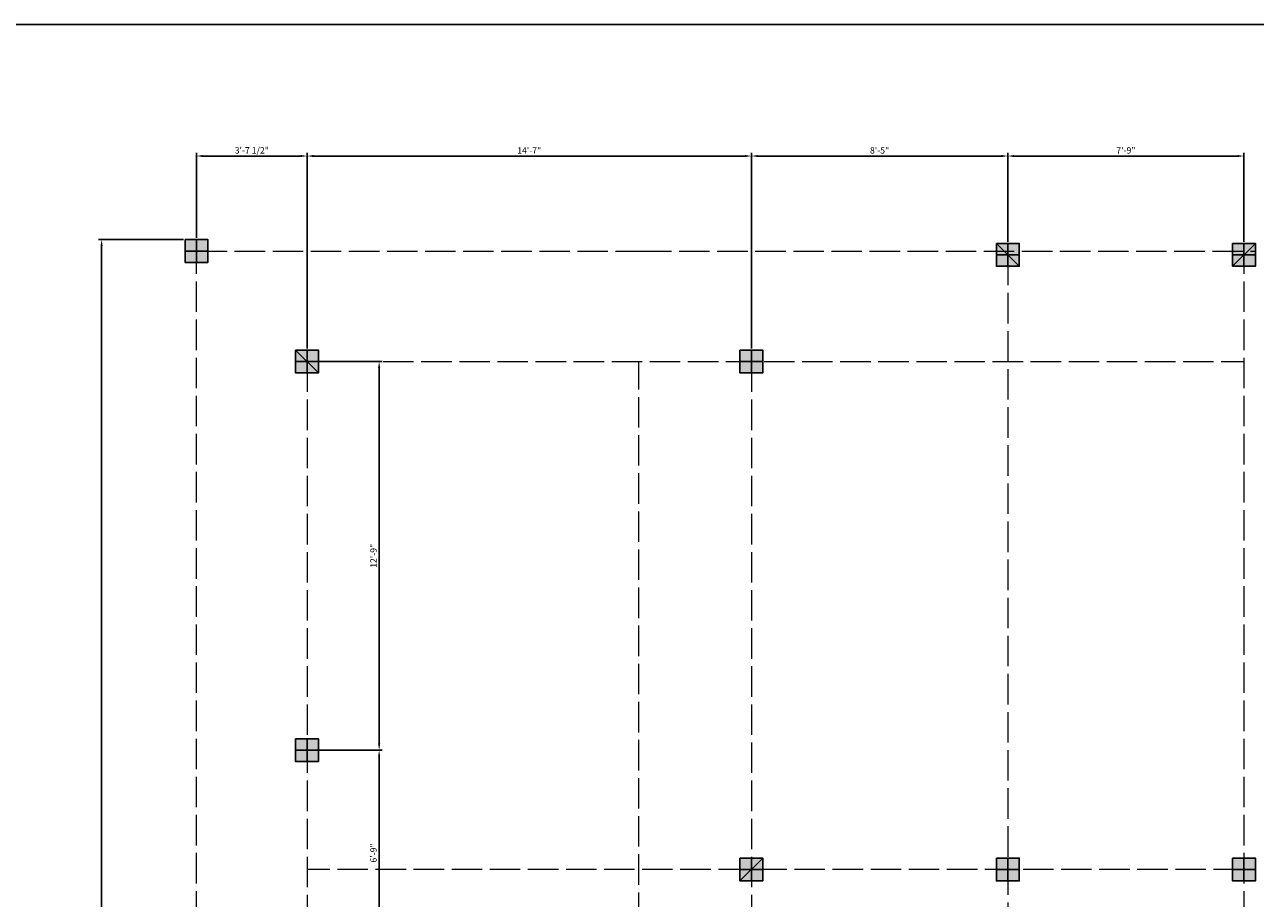
# Model space of a CAD drawing. Units: inches. Extents: x 2163 to 7246, y 928 to 2098.
# Tile 9 of 15: x 2706 to 3191, y 1754 to 2098. Entities that reach past the tile are written whole.
import ezdxf

# ---------------------------------------------------------------- set-up
doc = ezdxf.new("R2010")
doc.units = ezdxf.units.IN
doc.linetypes.add('ACAD_ISO02W100', pattern=[15, 12, -3])
for name, color, linetype, lineweight in [('A-ANNO-DIMS', 4, 'Continuous', 18), ('A-ANNO-TTLB', 7, 'Continuous', 30), ('A-COLS', 41, 'Continuous', 30), ('A-GRID', 1, 'ACAD_ISO02W100', 18)]:
    doc.layers.add(name, color=color, linetype=linetype, lineweight=lineweight)
doc.layers.add('A-COLS-PATT', color=51, linetype='Continuous', lineweight=9, true_color=0xf8f6b0)
doc.styles.get("Standard").update_dxf_attribs({"font": 'arial.ttf'})
doc.dimstyles.new('ISO-25', dxfattribs={"dimtxt": 2.5, "dimasz": 2.5, "dimexe": 1.25, "dimexo": 0.625, "dimtad": 1, "dimdec": 0, "dimlunit": 3, "dimtxsty": 'Standard', "dimcen": 2.5, "dimadec": 0, "dimazin": 0, "dimtfac": 1, "dimtdec": 0, "dimtmove": 0, "dimatfit": 3, "dimfxl": 1, "dimarcsym": 0})

# ---------------------------------------------------------------- blocks, each defined once
blk = doc.blocks.new('COL-9X9-CENTERED')
for p, q in [((4.5, 9), (4.5, 0)), ((0, 4.5), (9, 4.5))]:
    blk.add_line(p, q)
blk.add_lwpolyline([(0, 9), (9, 9), (9, 0), (0, 0)], close=True)
blk = doc.blocks.new('*D80')
at = {"layer": 'A-ANNO-DIMS', "color": 0, "lineweight": -2, "transparency": 16777216}
for p, q in [((2768.6, 2013.57), (2735.07, 2013.57)), ((2736.32, 2011.07), (2736.32, 1413.07)), ((2768.6, 1410.57), (2735.07, 1410.57))]:
    blk.add_line(p, q, dxfattribs=at)
at = {"layer": 'A-ANNO-DIMS', "color": 0, "transparency": 16777216}
for points in [[(2735.91, 2011.07), (2736.74, 2011.07), (2736.32, 2013.57)], [(2735.91, 1413.07), (2736.74, 1413.07), (2736.32, 1410.57)]]:
    blk.add_solid(points, dxfattribs=at)
at = {"layer": 'Defpoints', "color": 0, "transparency": 16777216}
for p in [(2769.22, 2013.57), (2736.32, 1410.57), (2769.22, 1410.57)]:
    blk.add_point(p, dxfattribs=at)
at = {"layer": 'A-ANNO-DIMS', "color": 0, "transparency": 16777216, "insert": (2734.42, 1712.07), "char_height": 2.5, "attachment_point": 5, "rotation": 90}
blk.add_mtext('50\'-3"', dxfattribs=at)
blk = doc.blocks.new('*D81')
at = {"layer": 'A-ANNO-DIMS', "color": 0, "lineweight": -2, "transparency": 16777216}
for p, q in [((2773.72, 2014.2), (2773.72, 2047.72)), ((2776.22, 2046.47), (2814.72, 2046.47)), ((2817.22, 1970.7), (2817.22, 2047.72))]:
    blk.add_line(p, q, dxfattribs=at)
at = {"layer": 'A-ANNO-DIMS', "color": 0, "transparency": 16777216}
for points in [[(2776.22, 2046.89), (2776.22, 2046.06), (2773.72, 2046.47)], [(2814.72, 2046.89), (2814.72, 2046.06), (2817.22, 2046.47)]]:
    blk.add_solid(points, dxfattribs=at)
at = {"layer": 'Defpoints', "color": 0, "transparency": 16777216}
for p in [(2817.22, 2046.47), (2773.72, 2013.57), (2817.22, 1970.07)]:
    blk.add_point(p, dxfattribs=at)
at = {"layer": 'A-ANNO-DIMS', "color": 0, "transparency": 16777216, "insert": (2795.47, 2048.39), "char_height": 2.5, "attachment_point": 5}
blk.add_mtext('3\'-7 1/2"', dxfattribs=at)
blk = doc.blocks.new('*D82')
at = {"layer": 'A-ANNO-DIMS', "color": 0, "lineweight": -2, "transparency": 16777216}
for p, q in [((2817.22, 1970.7), (2817.22, 2047.72)), ((2819.72, 2046.47), (2989.72, 2046.47)), ((2992.22, 1970.7), (2992.22, 2047.72))]:
    blk.add_line(p, q, dxfattribs=at)
at = {"layer": 'A-ANNO-DIMS', "color": 0, "transparency": 16777216}
for points in [[(2819.72, 2046.89), (2819.72, 2046.06), (2817.22, 2046.47)], [(2989.72, 2046.89), (2989.72, 2046.06), (2992.22, 2046.47)]]:
    blk.add_solid(points, dxfattribs=at)
at = {"layer": 'Defpoints', "color": 0, "transparency": 16777216}
for p in [(2992.22, 2046.47), (2817.22, 1970.07), (2992.22, 1970.07)]:
    blk.add_point(p, dxfattribs=at)
at = {"layer": 'A-ANNO-DIMS', "color": 0, "transparency": 16777216, "insert": (2904.72, 2048.35), "char_height": 2.5, "attachment_point": 5}
blk.add_mtext('14\'-7"', dxfattribs=at)
blk = doc.blocks.new('*D84')
at = {"layer": 'A-ANNO-DIMS', "color": 0, "lineweight": -2, "transparency": 16777216}
for p, q in [((2992.22, 1970.7), (2992.22, 2047.72)), ((2994.72, 2046.47), (3090.72, 2046.47)), ((3093.22, 2012.7), (3093.22, 2047.72))]:
    blk.add_line(p, q, dxfattribs=at)
at = {"layer": 'A-ANNO-DIMS', "color": 0, "transparency": 16777216}
for points in [[(2994.72, 2046.89), (2994.72, 2046.06), (2992.22, 2046.47)], [(3090.72, 2046.89), (3090.72, 2046.06), (3093.22, 2046.47)]]:
    blk.add_solid(points, dxfattribs=at)
at = {"layer": 'Defpoints', "color": 0, "transparency": 16777216}
for p in [(3093.22, 2046.47), (3093.22, 2012.07), (2992.22, 1970.07)]:
    blk.add_point(p, dxfattribs=at)
at = {"layer": 'A-ANNO-DIMS', "color": 0, "transparency": 16777216, "insert": (3042.72, 2048.37), "char_height": 2.5, "attachment_point": 5}
blk.add_mtext('8\'-5"', dxfattribs=at)
blk = doc.blocks.new('*D85')
at = {"layer": 'A-ANNO-DIMS', "color": 0, "lineweight": -2, "transparency": 16777216}
for p, q in [((3093.22, 2012.7), (3093.22, 2047.72)), ((3095.72, 2046.47), (3183.72, 2046.47)), ((3186.22, 2012.7), (3186.22, 2047.72))]:
    blk.add_line(p, q, dxfattribs=at)
at = {"layer": 'A-ANNO-DIMS', "color": 0, "transparency": 16777216}
for points in [[(3095.72, 2046.89), (3095.72, 2046.06), (3093.22, 2046.47)], [(3183.72, 2046.89), (3183.72, 2046.06), (3186.22, 2046.47)]]:
    blk.add_solid(points, dxfattribs=at)
at = {"layer": 'Defpoints', "color": 0, "transparency": 16777216}
for p in [(3186.22, 2046.47), (3093.22, 2012.07), (3186.22, 2012.07)]:
    blk.add_point(p, dxfattribs=at)
at = {"layer": 'A-ANNO-DIMS', "color": 0, "transparency": 16777216, "insert": (3139.72, 2048.37), "char_height": 2.5, "attachment_point": 5}
blk.add_mtext('7\'-9"', dxfattribs=at)
blk = doc.blocks.new('*D90')
at = {"layer": 'A-ANNO-DIMS', "color": 0, "lineweight": -2, "transparency": 16777216}
for p, q in [((2813.35, 1965.57), (2846.87, 1965.57)), ((2845.62, 1963.07), (2845.62, 1815.07)), ((2813.35, 1812.57), (2846.87, 1812.57))]:
    blk.add_line(p, q, dxfattribs=at)
at = {"layer": 'A-ANNO-DIMS', "color": 0, "transparency": 16777216}
for points in [[(2845.21, 1963.07), (2846.04, 1963.07), (2845.62, 1965.57)], [(2845.21, 1815.07), (2846.04, 1815.07), (2845.62, 1812.57)]]:
    blk.add_solid(points, dxfattribs=at)
at = {"layer": 'Defpoints', "color": 0, "transparency": 16777216}
for p in [(2812.72, 1965.57), (2812.72, 1812.57), (2845.62, 1812.57)]:
    blk.add_point(p, dxfattribs=at)
at = {"layer": 'A-ANNO-DIMS', "color": 0, "transparency": 16777216, "insert": (2843.72, 1889.07), "char_height": 2.5, "attachment_point": 5, "rotation": 90}
blk.add_mtext('12\'-9"', dxfattribs=at)
blk = doc.blocks.new('*D91')
at = {"layer": 'A-ANNO-DIMS', "color": 0, "lineweight": -2, "transparency": 16777216}
for p, q in [((2813.35, 1812.57), (2846.87, 1812.57)), ((2845.62, 1810.07), (2845.62, 1734.07)), ((2813.35, 1731.57), (2846.87, 1731.57))]:
    blk.add_line(p, q, dxfattribs=at)
at = {"layer": 'A-ANNO-DIMS', "color": 0, "transparency": 16777216}
for points in [[(2845.21, 1810.07), (2846.04, 1810.07), (2845.62, 1812.57)], [(2845.21, 1734.07), (2846.04, 1734.07), (2845.62, 1731.57)]]:
    blk.add_solid(points, dxfattribs=at)
at = {"layer": 'Defpoints', "color": 0, "transparency": 16777216}
for p in [(2812.72, 1812.57), (2812.72, 1731.57), (2845.62, 1731.57)]:
    blk.add_point(p, dxfattribs=at)
at = {"layer": 'A-ANNO-DIMS', "color": 0, "transparency": 16777216, "insert": (2843.72, 1772.07), "char_height": 2.5, "attachment_point": 5, "rotation": 90}
blk.add_mtext('6\'-9"', dxfattribs=at)

msp = doc.modelspace()

# ---------------------------------------------------------------- hatches: boundary and pattern name
at = {"layer": 'A-COLS-PATT'}
h = msp.add_hatch(color=256, dxfattribs=at)
h.dxf.hatch_style = 1
h.paths.add_polyline_path([(2778.22, 2009.07), (2773.72, 2009.07), (2773.72, 2004.57), (2778.22, 2004.57)])
h.paths.add_polyline_path([(2778.22, 2013.57), (2773.72, 2013.57), (2773.72, 2009.07), (2778.22, 2009.07)])
h.paths.add_polyline_path([(2773.72, 2013.57), (2769.22, 2013.57), (2769.22, 2009.07), (2773.72, 2009.07)])
h.paths.add_polyline_path([(2773.72, 2009.07), (2769.22, 2009.07), (2769.22, 2004.57), (2773.72, 2004.57)])
h.paths.add_polyline_path([(2817.22, 1965.57), (2812.72, 1965.57), (2812.72, 1961.07), (2817.22, 1961.07)])
h.paths.add_polyline_path([(2817.22, 1970.07), (2812.72, 1970.07), (2817.22, 1965.57)])
h.paths.add_polyline_path([(2821.72, 1965.57), (2817.22, 1965.57), (2821.72, 1961.07)], flags=17)
h.paths.add_polyline_path([(2817.22, 1965.57), (2817.22, 1961.07), (2821.72, 1961.07)], flags=17)
h.paths.add_polyline_path([(2821.72, 1970.07), (2817.22, 1970.07), (2817.22, 1965.57), (2821.72, 1965.57)])
h.paths.add_polyline_path([(2812.72, 1970.07), (2812.72, 1965.57), (2817.22, 1965.57)], flags=17)
h.paths.add_polyline_path([(2992.22, 1970.07), (2987.72, 1970.07), (2987.72, 1965.57), (2992.22, 1965.57)])
h.paths.add_polyline_path([(2996.72, 1970.07), (2992.22, 1970.07), (2992.22, 1965.57), (2996.72, 1965.57)])
h.paths.add_polyline_path([(2996.72, 1965.57), (2992.22, 1965.57), (2992.22, 1961.07), (2996.72, 1961.07)])
h.paths.add_polyline_path([(2992.22, 1965.57), (2987.72, 1965.57), (2987.72, 1961.07), (2992.22, 1961.07)])
h.paths.add_polyline_path([(3097.72, 2012.07), (3093.22, 2012.07), (3093.22, 2009.07), (3097.72, 2009.07)])
h.paths.add_polyline_path([(3093.22, 2012.07), (3088.72, 2012.07), (3091.72, 2009.07), (3093.22, 2009.07)])
h.paths.add_polyline_path([(3091.72, 2009.07), (3088.72, 2009.07), (3088.72, 2007.57), (3093.22, 2007.57)])
h.paths.add_polyline_path([(3088.72, 2012.07), (3088.72, 2009.07), (3091.72, 2009.07)])
h.paths.add_polyline_path([(3097.72, 2009.07), (3093.22, 2009.07), (3093.22, 2007.57), (3097.72, 2007.57)])
h.paths.add_polyline_path([(3093.22, 2009.07), (3091.72, 2009.07), (3093.22, 2007.57)], flags=17)
h.paths.add_polyline_path([(3093.22, 2007.57), (3088.72, 2007.57), (3088.72, 2003.07), (3093.22, 2003.07)])
h.paths.add_polyline_path([(3093.22, 2007.57), (3093.22, 2003.07), (3097.72, 2003.07)])
h.paths.add_polyline_path([(3097.72, 2007.57), (3093.22, 2007.57), (3097.72, 2003.07)], flags=17)
h.paths.add_polyline_path([(3186.22, 2012.07), (3181.72, 2012.07), (3181.72, 2009.07), (3186.22, 2009.07)])
h.paths.add_polyline_path([(3190.72, 2012.07), (3186.22, 2012.07), (3186.22, 2009.07), (3187.72, 2009.07)])
h.paths.add_polyline_path([(3190.72, 2012.07), (3187.72, 2009.07), (3190.72, 2009.07)], flags=17)
h.paths.add_polyline_path([(3190.72, 2009.07), (3187.72, 2009.07), (3186.22, 2007.57), (3190.72, 2007.57)])
h.paths.add_polyline_path([(3187.72, 2009.07), (3186.22, 2009.07), (3186.22, 2007.57)], flags=17)
h.paths.add_polyline_path([(3186.22, 2009.07), (3181.72, 2009.07), (3181.72, 2007.57), (3186.22, 2007.57)])
h.paths.add_polyline_path([(3186.22, 2007.57), (3181.72, 2007.57), (3181.72, 2003.07)], flags=17)
h.paths.add_polyline_path([(3186.22, 2007.57), (3181.72, 2003.07), (3186.22, 2003.07)], flags=17)
h.paths.add_polyline_path([(3190.72, 2007.57), (3186.22, 2007.57), (3186.22, 2003.07), (3190.72, 2003.07)])
h.paths.add_polyline_path([(2817.22, 1812.57), (2812.72, 1812.57), (2812.72, 1808.07), (2817.22, 1808.07)])
h.paths.add_polyline_path([(2817.22, 1817.07), (2812.72, 1817.07), (2812.72, 1812.57), (2817.22, 1812.57)])
h.paths.add_polyline_path([(2821.72, 1817.07), (2817.22, 1817.07), (2817.22, 1812.57), (2821.72, 1812.57)])
h.paths.add_polyline_path([(2821.72, 1812.57), (2817.22, 1812.57), (2817.22, 1808.07), (2821.72, 1808.07)])
h.paths.add_polyline_path([(2821.72, 1736.07), (2817.22, 1736.07), (2817.22, 1731.57), (2821.72, 1731.57)])
h.paths.add_polyline_path([(2817.22, 1736.07), (2812.72, 1736.07), (2812.72, 1731.57), (2817.22, 1731.57)])
h.paths.add_polyline_path([(2817.22, 1731.57), (2812.72, 1731.57), (2812.72, 1727.07), (2817.22, 1727.07)])
h.paths.add_polyline_path([(2821.72, 1731.57), (2817.22, 1731.57), (2817.22, 1727.07), (2821.72, 1727.07)])
h.paths.add_polyline_path([(2992.22, 1765.57), (2987.72, 1761.07), (2992.22, 1761.07)], flags=17)
h.paths.add_polyline_path([(2992.22, 1765.57), (2987.72, 1765.57), (2987.72, 1761.07)])
h.paths.add_polyline_path([(2992.22, 1770.07), (2987.72, 1770.07), (2987.72, 1765.57), (2992.22, 1765.57)])
h.paths.add_polyline_path([(2996.72, 1770.07), (2992.22, 1770.07), (2992.22, 1765.57)])
h.paths.add_polyline_path([(2996.72, 1770.07), (2992.22, 1765.57), (2996.72, 1765.57)], flags=17)
h.paths.add_polyline_path([(2996.72, 1765.57), (2992.22, 1765.57), (2992.22, 1761.07), (2996.72, 1761.07)])
h.paths.add_polyline_path([(3097.72, 1770.07), (3093.22, 1770.07), (3093.22, 1765.57), (3097.72, 1765.57)])
h.paths.add_polyline_path([(3093.22, 1770.07), (3088.72, 1770.07), (3088.72, 1765.57), (3093.22, 1765.57)])
h.paths.add_polyline_path([(3093.22, 1765.57), (3088.72, 1765.57), (3088.72, 1761.07), (3093.22, 1761.07)])
h.paths.add_polyline_path([(3097.72, 1765.57), (3093.22, 1765.57), (3093.22, 1761.07), (3097.72, 1761.07)])
h.paths.add_polyline_path([(3186.22, 1770.07), (3181.72, 1770.07), (3181.72, 1765.57), (3186.22, 1765.57)])
h.paths.add_polyline_path([(3190.72, 1770.07), (3186.22, 1770.07), (3186.22, 1765.57), (3190.72, 1765.57)])
h.paths.add_polyline_path([(3190.72, 1765.57), (3186.22, 1765.57), (3186.22, 1761.07), (3190.72, 1761.07)])
h.paths.add_polyline_path([(3186.22, 1765.57), (3181.72, 1765.57), (3181.72, 1761.07), (3186.22, 1761.07)])
h.paths.add_polyline_path([(2946.22, 1626.57), (2941.72, 1626.57), (2941.72, 1622.07), (2946.22, 1622.07)])
h.paths.add_polyline_path([(2946.22, 1631.07), (2941.72, 1631.07), (2941.72, 1626.57), (2946.22, 1626.57)])
h.paths.add_polyline_path([(2950.72, 1631.07), (2947.91, 1631.07), (2947.91, 1626.57), (2950.72, 1626.57)])
h.paths.add_polyline_path([(2947.91, 1631.07), (2946.22, 1631.07), (2946.22, 1626.57), (2947.91, 1626.57)])
h.paths.add_polyline_path([(2947.91, 1626.57), (2946.22, 1626.57), (2946.22, 1622.07), (2947.91, 1622.07)])
h.paths.add_polyline_path([(2950.72, 1626.57), (2947.91, 1626.57), (2947.91, 1622.07), (2950.72, 1622.07)])
h.paths.add_polyline_path([(2821.72, 1626.57), (2817.22, 1626.57), (2817.22, 1622.07), (2821.72, 1622.07)])
h.paths.add_polyline_path([(2821.72, 1631.07), (2817.22, 1626.57), (2821.72, 1626.57)])
h.paths.add_polyline_path([(2821.72, 1631.07), (2817.22, 1631.07), (2817.22, 1626.57)], flags=17)
h.paths.add_polyline_path([(2817.22, 1631.07), (2812.72, 1631.07), (2812.72, 1626.57), (2817.22, 1626.57)])
h.paths.add_polyline_path([(2817.22, 1626.57), (2812.72, 1626.57), (2812.72, 1622.07)], flags=17)
h.paths.add_polyline_path([(2817.22, 1626.57), (2812.72, 1622.07), (2817.22, 1622.07)])
h.paths.add_polyline_path([(3190.72, 1612.57), (3186.22, 1612.57), (3186.22, 1608.07), (3190.72, 1608.07)])
h.paths.add_polyline_path([(3186.22, 1612.57), (3181.72, 1608.07), (3186.22, 1608.07)], flags=17)
h.paths.add_polyline_path([(3186.22, 1612.57), (3181.72, 1612.57), (3181.72, 1608.07)], flags=17)
h.paths.add_polyline_path([(3186.22, 1617.07), (3181.72, 1617.07), (3181.72, 1612.57), (3186.22, 1612.57)])
h.paths.add_polyline_path([(3190.72, 1617.07), (3186.22, 1617.07), (3186.22, 1612.57)], flags=17)
h.paths.add_polyline_path([(3190.72, 1617.07), (3186.22, 1612.57), (3190.72, 1612.57)], flags=17)
h.paths.add_polyline_path([(2950.72, 1459.57), (2946.22, 1459.57), (2946.22, 1455.07), (2950.72, 1455.07)])
h.paths.add_polyline_path([(2946.22, 1459.57), (2941.72, 1455.07), (2946.22, 1455.07)])
h.paths.add_polyline_path([(2946.22, 1459.57), (2941.72, 1459.57), (2941.72, 1455.07)])
h.paths.add_polyline_path([(2946.22, 1464.07), (2941.72, 1464.07), (2941.72, 1459.57), (2946.22, 1459.57)])
h.paths.add_polyline_path([(2947.91, 1464.07), (2946.22, 1464.07), (2946.22, 1459.57), (2947.91, 1461.26)])
h.paths.add_polyline_path([(2950.72, 1464.07), (2947.91, 1464.07), (2947.91, 1461.26)])
h.paths.add_polyline_path([(2950.72, 1464.07), (2947.91, 1461.26), (2947.91, 1459.57), (2950.72, 1459.57)])
h.paths.add_polyline_path([(2950.72, 1459.57), (2947.91, 1459.57), (2946.22, 1459.57), (2946.22, 1455.07), (2950.72, 1455.07)], flags=17)
h.paths.add_polyline_path([(2947.91, 1461.26), (2946.22, 1459.57), (2947.91, 1459.57)], flags=17)
h.paths.add_polyline_path([(2773.72, 1415.07), (2769.22, 1415.07), (2769.22, 1410.57), (2773.72, 1410.57)])
h.paths.add_polyline_path([(2778.22, 1415.07), (2773.72, 1415.07), (2773.72, 1410.57), (2778.22, 1410.57)])
h.paths.add_polyline_path([(2778.22, 1419.57), (2773.72, 1419.57), (2773.72, 1415.07), (2778.22, 1415.07)])
h.paths.add_polyline_path([(2773.72, 1419.57), (2769.22, 1419.57), (2769.22, 1415.07), (2773.72, 1415.07)])
h.paths.add_polyline_path([(2992.22, 1415.07), (2987.72, 1415.07), (2987.72, 1410.57), (2992.22, 1410.57)])
h.paths.add_polyline_path([(2992.22, 1419.57), (2987.72, 1419.57), (2987.72, 1415.07), (2992.22, 1415.07)])
h.paths.add_polyline_path([(2996.72, 1419.57), (2992.22, 1419.57), (2992.22, 1415.07), (2996.72, 1415.07)])
h.paths.add_polyline_path([(2992.22, 1415.07), (2992.22, 1410.57), (2996.72, 1410.57), (2996.72, 1415.07)])

# ---------------------------------------------------------------- linework, layer by layer
at = {"layer": 'A-ANNO-TTLB'}
msp.add_lwpolyline([(2162.62, 2098.21), (3633.38, 2098.21), (3633.38, 928.48), (2162.62, 928.48)], close=True, dxfattribs=at)
at = {"layer": 'A-COLS'}
for p, q in [((3097.72, 2003.07), (3088.72, 2012.07)), ((3181.72, 2003.07), (3190.72, 2012.07)), ((2821.72, 1961.07), (2812.72, 1970.07)), ((2821.72, 1817.07), (2821.72, 1808.07)), ((2996.72, 1770.07), (2987.72, 1761.07))]:
    msp.add_line(p, q, dxfattribs=at)
at = {"layer": 'A-GRID'}
for p, q in [((2773.72, 2009.07), (2773.72, 2013.57)), ((3186.22, 2012.07), (3186.22, 1415.07)), ((2773.72, 1415.07), (2773.72, 2009.07)), ((2773.72, 2009.07), (2948.77, 2009.07)), ((2948.77, 2009.07), (3190.72, 2009.07)), ((3093.22, 2007.57), (3093.22, 1415.07)), ((2817.22, 1965.57), (2817.22, 1415.07)), ((2817.22, 1965.57), (3186.22, 1965.57)), ((2947.91, 1459.57), (2947.91, 1965.57)), ((2992.22, 1965.57), (2992.22, 1415.07)), ((3186.22, 1765.57), (2817.22, 1765.57))]:
    msp.add_line(p, q, dxfattribs=at)

# ---------------------------------------------------------------- block references
at = {"layer": 'A-COLS'}
for p in [(2769.22, 2004.57), (3088.72, 2003.07), (3181.72, 2003.07), (2812.72, 1961.07), (2987.72, 1961.07), (2812.72, 1808.07), (2987.72, 1761.07), (3088.72, 1761.07), (3181.72, 1761.07)]:
    msp.add_blockref('COL-9X9-CENTERED', p, dxfattribs=at)

# ---------------------------------------------------------------- dimensions: what is measured, and where the dimension line sits
at = {"layer": 'A-ANNO-DIMS'}
for base, p1, p2, picture, middle in [((2817.22, 2046.47), (2773.72, 2013.57), (2817.22, 1970.07), '*D81', (2795.47, 2048.39)), ((2992.22, 2046.47), (2817.22, 1970.07), (2992.22, 1970.07), '*D82', (2904.72, 2048.35)), ((3093.22, 2046.47), (2992.22, 1970.07), (3093.22, 2012.07), '*D84', (3042.72, 2048.37)), ((3186.22, 2046.47), (3093.22, 2012.07), (3186.22, 2012.07), '*D85', (3139.72, 2048.37))]:
    dim = msp.add_linear_dim(base=base, p1=p1, p2=p2, dimstyle='ISO-25', override={"dimdec": 1, "dimlfac": 1, "dimrnd": 0, "dimzin": 1, "dimdsep": 46, "dimlunit": 4, "dimfrac": 2}, dxfattribs=at)
    dim.commit()
    dim.dimension.update_dxf_attribs({"geometry": picture, "text_midpoint": middle})
for base, p1, p2, angle, picture, middle in [((2736.32, 1410.57), (2769.22, 2013.57), (2769.22, 1410.57), 90, '*D80', (2734.42, 1712.07)), ((2845.62, 1812.57), (2812.72, 1965.57), (2812.72, 1812.57), 270, '*D90', (2843.72, 1889.07)), ((2845.62, 1731.57), (2812.72, 1812.57), (2812.72, 1731.57), 270, '*D91', (2843.72, 1772.07))]:
    dim = msp.add_linear_dim(base=base, p1=p1, p2=p2, angle=angle, dimstyle='ISO-25', override={"dimdec": 1, "dimlfac": 1, "dimrnd": 0, "dimzin": 1, "dimdsep": 46, "dimlunit": 4, "dimfrac": 2}, dxfattribs=at)
    dim.commit()
    dim.dimension.update_dxf_attribs({"geometry": picture, "text_midpoint": middle})

doc.saveas('drawing.dxf')
